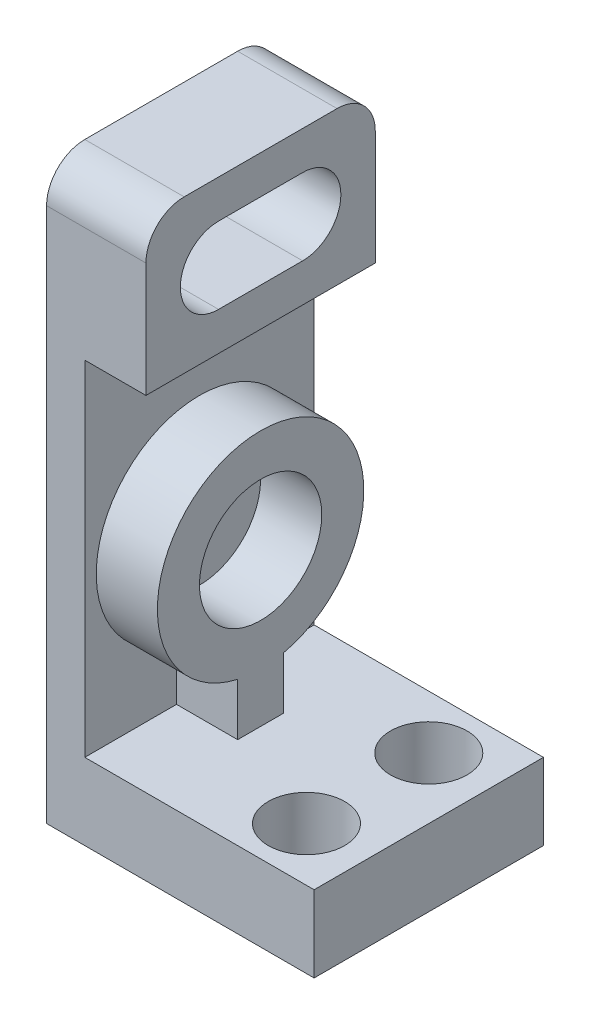
ISO-10303-21;
HEADER;
FILE_DESCRIPTION(('STEP AP214'),'2;1');
FILE_NAME('part.step','',(''),(''),'','','');
FILE_SCHEMA(('AUTOMOTIVE_DESIGN { 1 0 10303 214 1 1 1 1 }'));
ENDSEC;
DATA;
#1=APPLICATION_CONTEXT('core data for automotive mechanical design processes');
#2=APPLICATION_PROTOCOL_DEFINITION('international standard','automotive_design',2000,#1);
#3=PRODUCT_CONTEXT('',#1,'mechanical');
#4=PRODUCT('Part','Part','',(#3));
#5=PRODUCT_RELATED_PRODUCT_CATEGORY('part','',(#4));
#6=PRODUCT_DEFINITION_FORMATION('','',#4);
#7=PRODUCT_DEFINITION_CONTEXT('part definition',#1,'design');
#8=PRODUCT_DEFINITION('design','',#6,#7);
#9=PRODUCT_DEFINITION_SHAPE('','',#8);
#10=(LENGTH_UNIT() NAMED_UNIT(*) SI_UNIT(.MILLI.,.METRE.));
#11=(NAMED_UNIT(*) PLANE_ANGLE_UNIT() SI_UNIT($,.RADIAN.));
#12=(NAMED_UNIT(*) SI_UNIT($,.STERADIAN.) SOLID_ANGLE_UNIT());
#13=UNCERTAINTY_MEASURE_WITH_UNIT(LENGTH_MEASURE(1.E-05),#10,'distance_accuracy_value','');
#14=(GEOMETRIC_REPRESENTATION_CONTEXT(3) GLOBAL_UNCERTAINTY_ASSIGNED_CONTEXT((#13)) GLOBAL_UNIT_ASSIGNED_CONTEXT((#10,
#11,#12)) REPRESENTATION_CONTEXT('',''));
#15=CARTESIAN_POINT('',(0.,0.,0.));
#16=DIRECTION('',(0.,0.,1.));
#17=DIRECTION('',(1.,0.,0.));
#18=AXIS2_PLACEMENT_3D('',#15,#16,#17);
#19=CARTESIAN_POINT('',(0.,10.,-30.));
#20=DIRECTION('',(0.,1.,0.));
#21=DIRECTION('',(0.,0.,1.));
#22=AXIS2_PLACEMENT_3D('',#19,#20,#21);
#23=PLANE('',#22);
#24=CARTESIAN_POINT('',(27.,10.,-23.));
#25=DIRECTION('',(0.,1.,0.));
#26=DIRECTION('',(0.,0.,1.));
#27=AXIS2_PLACEMENT_3D('',#24,#25,#26);
#28=CIRCLE('',#27,5.);
#29=CARTESIAN_POINT('',(27.,10.,-18.));
#30=VERTEX_POINT('',#29);
#31=EDGE_CURVE('E263',#30,#30,#28,.T.);
#32=ORIENTED_EDGE('',*,*,#31,.F.);
#33=EDGE_LOOP('',(#32));
#34=FACE_BOUND('',#33,.T.);
#35=CARTESIAN_POINT('',(27.,10.,-7.));
#36=DIRECTION('',(0.,1.,0.));
#37=DIRECTION('',(0.,0.,1.));
#38=AXIS2_PLACEMENT_3D('',#35,#36,#37);
#39=CIRCLE('',#38,5.);
#40=CARTESIAN_POINT('',(27.,10.,-2.));
#41=VERTEX_POINT('',#40);
#42=EDGE_CURVE('E251',#41,#41,#39,.T.);
#43=ORIENTED_EDGE('',*,*,#42,.F.);
#44=EDGE_LOOP('',(#43));
#45=FACE_BOUND('',#44,.T.);
#46=DIRECTION('',(0.,0.,1.));
#47=VECTOR('',#46,1.);
#48=CARTESIAN_POINT('',(5.,10.,-30.));
#49=LINE('',#48,#47);
#50=CARTESIAN_POINT('',(5.,10.,-30.));
#51=VERTEX_POINT('',#50);
#52=CARTESIAN_POINT('',(5.,10.,-18.));
#53=VERTEX_POINT('',#52);
#54=EDGE_CURVE('E186',#51,#53,#49,.T.);
#55=ORIENTED_EDGE('',*,*,#54,.T.);
#56=DIRECTION('',(-1.,0.,0.));
#57=VECTOR('',#56,1.);
#58=CARTESIAN_POINT('',(13.,10.,-18.));
#59=LINE('',#58,#57);
#60=CARTESIAN_POINT('',(13.,10.,-18.));
#61=VERTEX_POINT('',#60);
#62=EDGE_CURVE('E169',#61,#53,#59,.T.);
#63=ORIENTED_EDGE('',*,*,#62,.F.);
#64=DIRECTION('',(0.,0.,-1.));
#65=VECTOR('',#64,1.);
#66=CARTESIAN_POINT('',(13.,10.,-12.));
#67=LINE('',#66,#65);
#68=CARTESIAN_POINT('',(13.,10.,-12.));
#69=VERTEX_POINT('',#68);
#70=EDGE_CURVE('E172',#69,#61,#67,.T.);
#71=ORIENTED_EDGE('',*,*,#70,.F.);
#72=DIRECTION('',(-1.,0.,0.));
#73=VECTOR('',#72,1.);
#74=CARTESIAN_POINT('',(13.,10.,-12.));
#75=LINE('',#74,#73);
#76=CARTESIAN_POINT('',(5.,10.,-12.));
#77=VERTEX_POINT('',#76);
#78=EDGE_CURVE('E371',#69,#77,#75,.T.);
#79=ORIENTED_EDGE('',*,*,#78,.T.);
#80=CARTESIAN_POINT('',(5.,10.,0.));
#81=VERTEX_POINT('',#80);
#82=EDGE_CURVE('E275',#77,#81,#49,.T.);
#83=ORIENTED_EDGE('',*,*,#82,.T.);
#84=DIRECTION('',(-1.,0.,0.));
#85=VECTOR('',#84,1.);
#86=CARTESIAN_POINT('',(0.,10.,0.));
#87=LINE('',#86,#85);
#88=CARTESIAN_POINT('',(35.,10.,0.));
#89=VERTEX_POINT('',#88);
#90=EDGE_CURVE('E288',#89,#81,#87,.T.);
#91=ORIENTED_EDGE('',*,*,#90,.F.);
#92=DIRECTION('',(0.,0.,1.));
#93=VECTOR('',#92,1.);
#94=CARTESIAN_POINT('',(35.,10.,-30.));
#95=LINE('',#94,#93);
#96=CARTESIAN_POINT('',(35.,10.,-30.));
#97=VERTEX_POINT('',#96);
#98=EDGE_CURVE('E50',#97,#89,#95,.T.);
#99=ORIENTED_EDGE('',*,*,#98,.F.);
#100=DIRECTION('',(-1.,0.,0.));
#101=VECTOR('',#100,1.);
#102=CARTESIAN_POINT('',(0.,10.,-30.));
#103=LINE('',#102,#101);
#104=EDGE_CURVE('E295',#97,#51,#103,.T.);
#105=ORIENTED_EDGE('',*,*,#104,.T.);
#106=EDGE_LOOP('',(#55,#63,#71,#79,#83,#91,#99,#105));
#107=FACE_BOUND('',#106,.T.);
#108=ADVANCED_FACE('F39',(#34,#45,#107),#23,.T.);
#109=CARTESIAN_POINT('',(0.,0.,-30.));
#110=DIRECTION('',(-1.,0.,0.));
#111=DIRECTION('',(0.,0.,1.));
#112=AXIS2_PLACEMENT_3D('',#109,#110,#111);
#113=PLANE('',#112);
#114=CARTESIAN_POINT('',(0.,65.,-9.5));
#115=DIRECTION('',(1.,0.,0.));
#116=DIRECTION('',(0.,0.,-1.));
#117=AXIS2_PLACEMENT_3D('',#114,#115,#116);
#118=CIRCLE('',#117,5.);
#119=CARTESIAN_POINT('',(0.,70.,-9.5));
#120=VERTEX_POINT('',#119);
#121=CARTESIAN_POINT('',(0.,60.,-9.5));
#122=VERTEX_POINT('',#121);
#123=EDGE_CURVE('E198',#120,#122,#118,.T.);
#124=ORIENTED_EDGE('',*,*,#123,.T.);
#125=DIRECTION('',(0.,0.,-1.));
#126=VECTOR('',#125,1.);
#127=CARTESIAN_POINT('',(0.,60.,-9.5));
#128=LINE('',#127,#126);
#129=CARTESIAN_POINT('',(0.,60.,-20.5));
#130=VERTEX_POINT('',#129);
#131=EDGE_CURVE('E200',#122,#130,#128,.T.);
#132=ORIENTED_EDGE('',*,*,#131,.T.);
#133=CARTESIAN_POINT('',(0.,65.,-20.5));
#134=DIRECTION('',(1.,0.,0.));
#135=DIRECTION('',(0.,0.,-1.));
#136=AXIS2_PLACEMENT_3D('',#133,#134,#135);
#137=CIRCLE('',#136,5.);
#138=CARTESIAN_POINT('',(0.,70.,-20.5));
#139=VERTEX_POINT('',#138);
#140=EDGE_CURVE('E65',#130,#139,#137,.T.);
#141=ORIENTED_EDGE('',*,*,#140,.T.);
#142=DIRECTION('',(0.,0.,1.));
#143=VECTOR('',#142,1.);
#144=CARTESIAN_POINT('',(0.,70.,-9.5));
#145=LINE('',#144,#143);
#146=EDGE_CURVE('E204',#139,#120,#145,.T.);
#147=ORIENTED_EDGE('',*,*,#146,.T.);
#148=EDGE_LOOP('',(#124,#132,#141,#147));
#149=FACE_BOUND('',#148,.T.);
#150=DIRECTION('',(0.,-1.,0.));
#151=VECTOR('',#150,1.);
#152=CARTESIAN_POINT('',(0.,0.,0.));
#153=LINE('',#152,#151);
#154=CARTESIAN_POINT('',(0.,70.,0.));
#155=VERTEX_POINT('',#154);
#156=CARTESIAN_POINT('',(0.,0.,0.));
#157=VERTEX_POINT('',#156);
#158=EDGE_CURVE('E278',#155,#157,#153,.T.);
#159=ORIENTED_EDGE('',*,*,#158,.F.);
#160=CARTESIAN_POINT('',(0.,70.,-5.));
#161=DIRECTION('',(1.,0.,0.));
#162=DIRECTION('',(0.,0.,1.));
#163=AXIS2_PLACEMENT_3D('',#160,#161,#162);
#164=CIRCLE('',#163,5.);
#165=CARTESIAN_POINT('',(0.,75.,-5.00000000000004));
#166=VERTEX_POINT('',#165);
#167=EDGE_CURVE('E249',#166,#155,#164,.T.);
#168=ORIENTED_EDGE('',*,*,#167,.F.);
#169=DIRECTION('',(0.,0.,1.));
#170=VECTOR('',#169,1.);
#171=CARTESIAN_POINT('',(0.,75.,-5.00000000000004));
#172=LINE('',#171,#170);
#173=CARTESIAN_POINT('',(0.,75.,-25.));
#174=VERTEX_POINT('',#173);
#175=EDGE_CURVE('E244',#174,#166,#172,.T.);
#176=ORIENTED_EDGE('',*,*,#175,.F.);
#177=CARTESIAN_POINT('',(0.,70.,-25.));
#178=DIRECTION('',(1.,0.,0.));
#179=DIRECTION('',(0.,0.,1.));
#180=AXIS2_PLACEMENT_3D('',#177,#178,#179);
#181=CIRCLE('',#180,5.);
#182=CARTESIAN_POINT('',(0.,70.,-30.));
#183=VERTEX_POINT('',#182);
#184=EDGE_CURVE('E243',#183,#174,#181,.T.);
#185=ORIENTED_EDGE('',*,*,#184,.F.);
#186=DIRECTION('',(0.,-1.,0.));
#187=VECTOR('',#186,1.);
#188=CARTESIAN_POINT('',(0.,0.,-30.));
#189=LINE('',#188,#187);
#190=CARTESIAN_POINT('',(0.,0.,-30.));
#191=VERTEX_POINT('',#190);
#192=EDGE_CURVE('E285',#183,#191,#189,.T.);
#193=ORIENTED_EDGE('',*,*,#192,.T.);
#194=DIRECTION('',(0.,0.,1.));
#195=VECTOR('',#194,1.);
#196=CARTESIAN_POINT('',(0.,0.,-30.));
#197=LINE('',#196,#195);
#198=EDGE_CURVE('E294',#191,#157,#197,.T.);
#199=ORIENTED_EDGE('',*,*,#198,.T.);
#200=EDGE_LOOP('',(#159,#168,#176,#185,#193,#199));
#201=FACE_BOUND('',#200,.T.);
#202=ADVANCED_FACE('F41',(#149,#201),#113,.T.);
#203=CARTESIAN_POINT('',(35.,0.,-30.));
#204=DIRECTION('',(1.,0.,0.));
#205=DIRECTION('',(0.,0.,-1.));
#206=AXIS2_PLACEMENT_3D('',#203,#204,#205);
#207=PLANE('',#206);
#208=DIRECTION('',(0.,1.,0.));
#209=VECTOR('',#208,1.);
#210=CARTESIAN_POINT('',(35.,0.,0.));
#211=LINE('',#210,#209);
#212=CARTESIAN_POINT('',(35.,0.,0.));
#213=VERTEX_POINT('',#212);
#214=EDGE_CURVE('E297',#213,#89,#211,.T.);
#215=ORIENTED_EDGE('',*,*,#214,.F.);
#216=DIRECTION('',(0.,0.,1.));
#217=VECTOR('',#216,1.);
#218=CARTESIAN_POINT('',(35.,0.,-30.));
#219=LINE('',#218,#217);
#220=CARTESIAN_POINT('',(35.,0.,-30.));
#221=VERTEX_POINT('',#220);
#222=EDGE_CURVE('E308',#221,#213,#219,.T.);
#223=ORIENTED_EDGE('',*,*,#222,.F.);
#224=DIRECTION('',(0.,1.,0.));
#225=VECTOR('',#224,1.);
#226=CARTESIAN_POINT('',(35.,0.,-30.));
#227=LINE('',#226,#225);
#228=EDGE_CURVE('E290',#221,#97,#227,.T.);
#229=ORIENTED_EDGE('',*,*,#228,.T.);
#230=ORIENTED_EDGE('',*,*,#98,.T.);
#231=EDGE_LOOP('',(#215,#223,#229,#230));
#232=FACE_BOUND('',#231,.T.);
#233=ADVANCED_FACE('F319',(#232),#207,.T.);
#234=CARTESIAN_POINT('',(0.,0.,-30.));
#235=DIRECTION('',(0.,-1.,0.));
#236=DIRECTION('',(0.,0.,-1.));
#237=AXIS2_PLACEMENT_3D('',#234,#235,#236);
#238=PLANE('',#237);
#239=CARTESIAN_POINT('',(27.,0.,-23.));
#240=DIRECTION('',(0.,-1.,0.));
#241=DIRECTION('',(0.,0.,-1.));
#242=AXIS2_PLACEMENT_3D('',#239,#240,#241);
#243=CIRCLE('',#242,5.);
#244=CARTESIAN_POINT('',(27.,0.,-28.));
#245=VERTEX_POINT('',#244);
#246=EDGE_CURVE('E277',#245,#245,#243,.T.);
#247=ORIENTED_EDGE('',*,*,#246,.F.);
#248=EDGE_LOOP('',(#247));
#249=FACE_BOUND('',#248,.T.);
#250=CARTESIAN_POINT('',(27.,0.,-7.));
#251=DIRECTION('',(0.,-1.,0.));
#252=DIRECTION('',(0.,0.,-1.));
#253=AXIS2_PLACEMENT_3D('',#250,#251,#252);
#254=CIRCLE('',#253,5.);
#255=CARTESIAN_POINT('',(27.,0.,-12.));
#256=VERTEX_POINT('',#255);
#257=EDGE_CURVE('E266',#256,#256,#254,.T.);
#258=ORIENTED_EDGE('',*,*,#257,.F.);
#259=EDGE_LOOP('',(#258));
#260=FACE_BOUND('',#259,.T.);
#261=DIRECTION('',(1.,0.,0.));
#262=VECTOR('',#261,1.);
#263=CARTESIAN_POINT('',(0.,0.,0.));
#264=LINE('',#263,#262);
#265=EDGE_CURVE('E300',#157,#213,#264,.T.);
#266=ORIENTED_EDGE('',*,*,#265,.F.);
#267=ORIENTED_EDGE('',*,*,#198,.F.);
#268=DIRECTION('',(1.,0.,0.));
#269=VECTOR('',#268,1.);
#270=CARTESIAN_POINT('',(0.,0.,-30.));
#271=LINE('',#270,#269);
#272=EDGE_CURVE('E282',#191,#221,#271,.T.);
#273=ORIENTED_EDGE('',*,*,#272,.T.);
#274=ORIENTED_EDGE('',*,*,#222,.T.);
#275=EDGE_LOOP('',(#266,#267,#273,#274));
#276=FACE_BOUND('',#275,.T.);
#277=ADVANCED_FACE('F316',(#249,#260,#276),#238,.T.);
#278=CARTESIAN_POINT('',(0.,0.,-30.));
#279=DIRECTION('',(0.,0.,-1.));
#280=DIRECTION('',(-1.,0.,0.));
#281=AXIS2_PLACEMENT_3D('',#278,#279,#280);
#282=PLANE('',#281);
#283=ORIENTED_EDGE('',*,*,#192,.F.);
#284=DIRECTION('',(1.,0.,0.));
#285=VECTOR('',#284,1.);
#286=CARTESIAN_POINT('',(0.,70.,-30.));
#287=LINE('',#286,#285);
#288=CARTESIAN_POINT('',(13.,70.,-30.));
#289=VERTEX_POINT('',#288);
#290=EDGE_CURVE('E256',#183,#289,#287,.T.);
#291=ORIENTED_EDGE('',*,*,#290,.T.);
#292=DIRECTION('',(0.,1.,0.));
#293=VECTOR('',#292,1.);
#294=CARTESIAN_POINT('',(13.,55.,-30.));
#295=LINE('',#294,#293);
#296=CARTESIAN_POINT('',(13.,55.,-30.));
#297=VERTEX_POINT('',#296);
#298=EDGE_CURVE('E229',#297,#289,#295,.T.);
#299=ORIENTED_EDGE('',*,*,#298,.F.);
#300=DIRECTION('',(1.,0.,0.));
#301=VECTOR('',#300,1.);
#302=CARTESIAN_POINT('',(0.,55.,-30.));
#303=LINE('',#302,#301);
#304=CARTESIAN_POINT('',(5.,55.,-30.));
#305=VERTEX_POINT('',#304);
#306=EDGE_CURVE('E257',#305,#297,#303,.T.);
#307=ORIENTED_EDGE('',*,*,#306,.F.);
#308=DIRECTION('',(0.,1.,0.));
#309=VECTOR('',#308,1.);
#310=CARTESIAN_POINT('',(5.,10.,-30.));
#311=LINE('',#310,#309);
#312=EDGE_CURVE('E267',#51,#305,#311,.T.);
#313=ORIENTED_EDGE('',*,*,#312,.F.);
#314=ORIENTED_EDGE('',*,*,#104,.F.);
#315=ORIENTED_EDGE('',*,*,#228,.F.);
#316=ORIENTED_EDGE('',*,*,#272,.F.);
#317=EDGE_LOOP('',(#283,#291,#299,#307,#313,#314,#315,#316));
#318=FACE_BOUND('',#317,.T.);
#319=ADVANCED_FACE('F317',(#318),#282,.T.);
#320=CARTESIAN_POINT('',(0.,0.,0.));
#321=DIRECTION('',(0.,0.,-1.));
#322=DIRECTION('',(-1.,0.,0.));
#323=AXIS2_PLACEMENT_3D('',#320,#321,#322);
#324=PLANE('',#323);
#325=ORIENTED_EDGE('',*,*,#158,.T.);
#326=ORIENTED_EDGE('',*,*,#265,.T.);
#327=ORIENTED_EDGE('',*,*,#214,.T.);
#328=ORIENTED_EDGE('',*,*,#90,.T.);
#329=DIRECTION('',(0.,1.,0.));
#330=VECTOR('',#329,1.);
#331=CARTESIAN_POINT('',(5.,10.,0.));
#332=LINE('',#331,#330);
#333=CARTESIAN_POINT('',(5.,55.,0.));
#334=VERTEX_POINT('',#333);
#335=EDGE_CURVE('E272',#81,#334,#332,.T.);
#336=ORIENTED_EDGE('',*,*,#335,.T.);
#337=DIRECTION('',(1.,0.,0.));
#338=VECTOR('',#337,1.);
#339=CARTESIAN_POINT('',(0.,55.,0.));
#340=LINE('',#339,#338);
#341=CARTESIAN_POINT('',(13.,55.,0.));
#342=VERTEX_POINT('',#341);
#343=EDGE_CURVE('E246',#334,#342,#340,.T.);
#344=ORIENTED_EDGE('',*,*,#343,.T.);
#345=DIRECTION('',(0.,-1.,0.));
#346=VECTOR('',#345,1.);
#347=CARTESIAN_POINT('',(13.,55.,0.));
#348=LINE('',#347,#346);
#349=CARTESIAN_POINT('',(13.,70.,0.));
#350=VERTEX_POINT('',#349);
#351=EDGE_CURVE('E220',#350,#342,#348,.T.);
#352=ORIENTED_EDGE('',*,*,#351,.F.);
#353=DIRECTION('',(1.,0.,0.));
#354=VECTOR('',#353,1.);
#355=CARTESIAN_POINT('',(0.,70.,0.));
#356=LINE('',#355,#354);
#357=EDGE_CURVE('E253',#155,#350,#356,.T.);
#358=ORIENTED_EDGE('',*,*,#357,.F.);
#359=EDGE_LOOP('',(#325,#326,#327,#328,#336,#344,#352,#358));
#360=FACE_BOUND('',#359,.T.);
#361=ADVANCED_FACE('F327',(#360),#324,.F.);
#362=CARTESIAN_POINT('',(5.,10.,-30.));
#363=DIRECTION('',(1.,0.,0.));
#364=DIRECTION('',(0.,0.,-1.));
#365=AXIS2_PLACEMENT_3D('',#362,#363,#364);
#366=PLANE('',#365);
#367=CARTESIAN_POINT('',(5.,30.,-15.));
#368=DIRECTION('',(1.,0.,0.));
#369=DIRECTION('',(0.,0.,-1.));
#370=AXIS2_PLACEMENT_3D('',#367,#368,#369);
#371=CIRCLE('',#370,13.5);
#372=CARTESIAN_POINT('',(5.,16.8375534189118,-18.));
#373=VERTEX_POINT('',#372);
#374=CARTESIAN_POINT('',(5.,16.8375534189118,-12.));
#375=VERTEX_POINT('',#374);
#376=EDGE_CURVE('E363',#373,#375,#371,.T.);
#377=ORIENTED_EDGE('',*,*,#376,.F.);
#378=DIRECTION('',(0.,1.,0.));
#379=VECTOR('',#378,1.);
#380=CARTESIAN_POINT('',(5.,16.8375534189118,-18.));
#381=LINE('',#380,#379);
#382=EDGE_CURVE('E360',#53,#373,#381,.T.);
#383=ORIENTED_EDGE('',*,*,#382,.F.);
#384=ORIENTED_EDGE('',*,*,#54,.F.);
#385=ORIENTED_EDGE('',*,*,#312,.T.);
#386=DIRECTION('',(0.,0.,1.));
#387=VECTOR('',#386,1.);
#388=CARTESIAN_POINT('',(5.,55.,-30.));
#389=LINE('',#388,#387);
#390=EDGE_CURVE('E280',#305,#334,#389,.T.);
#391=ORIENTED_EDGE('',*,*,#390,.T.);
#392=ORIENTED_EDGE('',*,*,#335,.F.);
#393=ORIENTED_EDGE('',*,*,#82,.F.);
#394=DIRECTION('',(0.,-1.,0.));
#395=VECTOR('',#394,1.);
#396=CARTESIAN_POINT('',(5.,16.8375534189118,-12.));
#397=LINE('',#396,#395);
#398=EDGE_CURVE('E184',#375,#77,#397,.T.);
#399=ORIENTED_EDGE('',*,*,#398,.F.);
#400=EDGE_LOOP('',(#377,#383,#384,#385,#391,#392,#393,#399));
#401=FACE_BOUND('',#400,.T.);
#402=ADVANCED_FACE('F357',(#401),#366,.T.);
#403=CARTESIAN_POINT('',(27.,-20.,-7.));
#404=DIRECTION('',(0.,1.,0.));
#405=DIRECTION('',(0.,0.,1.));
#406=AXIS2_PLACEMENT_3D('',#403,#404,#405);
#407=CYLINDRICAL_SURFACE('',#406,5.);
#408=ORIENTED_EDGE('',*,*,#257,.T.);
#409=EDGE_LOOP('',(#408));
#410=FACE_BOUND('',#409,.T.);
#411=ORIENTED_EDGE('',*,*,#42,.T.);
#412=EDGE_LOOP('',(#411));
#413=FACE_BOUND('',#412,.T.);
#414=ADVANCED_FACE('F400',(#410,#413),#407,.F.);
#415=CARTESIAN_POINT('',(27.,-20.,-23.));
#416=DIRECTION('',(0.,1.,0.));
#417=DIRECTION('',(0.,0.,1.));
#418=AXIS2_PLACEMENT_3D('',#415,#416,#417);
#419=CYLINDRICAL_SURFACE('',#418,5.);
#420=ORIENTED_EDGE('',*,*,#246,.T.);
#421=EDGE_LOOP('',(#420));
#422=FACE_BOUND('',#421,.T.);
#423=ORIENTED_EDGE('',*,*,#31,.T.);
#424=EDGE_LOOP('',(#423));
#425=FACE_BOUND('',#424,.T.);
#426=ADVANCED_FACE('F311',(#422,#425),#419,.F.);
#427=CARTESIAN_POINT('',(0.,55.,0.));
#428=DIRECTION('',(0.,-1.,0.));
#429=DIRECTION('',(0.,0.,-1.));
#430=AXIS2_PLACEMENT_3D('',#427,#428,#429);
#431=PLANE('',#430);
#432=ORIENTED_EDGE('',*,*,#390,.F.);
#433=ORIENTED_EDGE('',*,*,#306,.T.);
#434=DIRECTION('',(0.,0.,-1.));
#435=VECTOR('',#434,1.);
#436=CARTESIAN_POINT('',(13.,55.,0.));
#437=LINE('',#436,#435);
#438=EDGE_CURVE('E228',#342,#297,#437,.T.);
#439=ORIENTED_EDGE('',*,*,#438,.F.);
#440=ORIENTED_EDGE('',*,*,#343,.F.);
#441=EDGE_LOOP('',(#432,#433,#439,#440));
#442=FACE_BOUND('',#441,.T.);
#443=ADVANCED_FACE('F355',(#442),#431,.T.);
#444=CARTESIAN_POINT('',(0.,70.,-5.));
#445=DIRECTION('',(1.,0.,0.));
#446=DIRECTION('',(0.,0.,-1.));
#447=AXIS2_PLACEMENT_3D('',#444,#445,#446);
#448=CYLINDRICAL_SURFACE('',#447,5.);
#449=ORIENTED_EDGE('',*,*,#357,.T.);
#450=CARTESIAN_POINT('',(13.,70.,-5.));
#451=DIRECTION('',(1.,0.,0.));
#452=DIRECTION('',(0.,0.,1.));
#453=AXIS2_PLACEMENT_3D('',#450,#451,#452);
#454=CIRCLE('',#453,5.);
#455=CARTESIAN_POINT('',(13.,75.,-5.00000000000004));
#456=VERTEX_POINT('',#455);
#457=EDGE_CURVE('E236',#456,#350,#454,.T.);
#458=ORIENTED_EDGE('',*,*,#457,.F.);
#459=DIRECTION('',(1.,0.,0.));
#460=VECTOR('',#459,1.);
#461=CARTESIAN_POINT('',(0.,75.,-5.00000000000004));
#462=LINE('',#461,#460);
#463=EDGE_CURVE('E255',#166,#456,#462,.T.);
#464=ORIENTED_EDGE('',*,*,#463,.F.);
#465=ORIENTED_EDGE('',*,*,#167,.T.);
#466=EDGE_LOOP('',(#449,#458,#464,#465));
#467=FACE_BOUND('',#466,.T.);
#468=ADVANCED_FACE('F346',(#467),#448,.T.);
#469=CARTESIAN_POINT('',(0.,75.,-5.00000000000004));
#470=DIRECTION('',(0.,1.,0.));
#471=DIRECTION('',(0.,0.,1.));
#472=AXIS2_PLACEMENT_3D('',#469,#470,#471);
#473=PLANE('',#472);
#474=ORIENTED_EDGE('',*,*,#463,.T.);
#475=DIRECTION('',(0.,0.,1.));
#476=VECTOR('',#475,1.);
#477=CARTESIAN_POINT('',(13.,75.,-5.00000000000004));
#478=LINE('',#477,#476);
#479=CARTESIAN_POINT('',(13.,75.,-25.));
#480=VERTEX_POINT('',#479);
#481=EDGE_CURVE('E231',#480,#456,#478,.T.);
#482=ORIENTED_EDGE('',*,*,#481,.F.);
#483=DIRECTION('',(1.,0.,0.));
#484=VECTOR('',#483,1.);
#485=CARTESIAN_POINT('',(0.,75.,-25.));
#486=LINE('',#485,#484);
#487=EDGE_CURVE('E258',#174,#480,#486,.T.);
#488=ORIENTED_EDGE('',*,*,#487,.F.);
#489=ORIENTED_EDGE('',*,*,#175,.T.);
#490=EDGE_LOOP('',(#474,#482,#488,#489));
#491=FACE_BOUND('',#490,.T.);
#492=ADVANCED_FACE('F347',(#491),#473,.T.);
#493=CARTESIAN_POINT('',(0.,70.,-25.));
#494=DIRECTION('',(1.,0.,0.));
#495=DIRECTION('',(0.,0.,-1.));
#496=AXIS2_PLACEMENT_3D('',#493,#494,#495);
#497=CYLINDRICAL_SURFACE('',#496,5.);
#498=ORIENTED_EDGE('',*,*,#487,.T.);
#499=CARTESIAN_POINT('',(13.,70.,-25.));
#500=DIRECTION('',(1.,0.,0.));
#501=DIRECTION('',(0.,0.,1.));
#502=AXIS2_PLACEMENT_3D('',#499,#500,#501);
#503=CIRCLE('',#502,5.);
#504=EDGE_CURVE('E234',#289,#480,#503,.T.);
#505=ORIENTED_EDGE('',*,*,#504,.F.);
#506=ORIENTED_EDGE('',*,*,#290,.F.);
#507=ORIENTED_EDGE('',*,*,#184,.T.);
#508=EDGE_LOOP('',(#498,#505,#506,#507));
#509=FACE_BOUND('',#508,.T.);
#510=ADVANCED_FACE('F337',(#509),#497,.T.);
#511=CARTESIAN_POINT('',(13.,70.,-5.));
#512=DIRECTION('',(-1.,0.,0.));
#513=DIRECTION('',(0.,0.,1.));
#514=AXIS2_PLACEMENT_3D('',#511,#512,#513);
#515=PLANE('',#514);
#516=DIRECTION('',(0.,0.,-1.));
#517=VECTOR('',#516,1.);
#518=CARTESIAN_POINT('',(13.,60.,-9.5));
#519=LINE('',#518,#517);
#520=CARTESIAN_POINT('',(13.,60.,-9.5));
#521=VERTEX_POINT('',#520);
#522=CARTESIAN_POINT('',(13.,60.,-20.5));
#523=VERTEX_POINT('',#522);
#524=EDGE_CURVE('E193',#521,#523,#519,.T.);
#525=ORIENTED_EDGE('',*,*,#524,.F.);
#526=CARTESIAN_POINT('',(13.,65.,-9.5));
#527=DIRECTION('',(1.,0.,0.));
#528=DIRECTION('',(0.,0.,-1.));
#529=AXIS2_PLACEMENT_3D('',#526,#527,#528);
#530=CIRCLE('',#529,5.);
#531=CARTESIAN_POINT('',(13.,70.,-9.5));
#532=VERTEX_POINT('',#531);
#533=EDGE_CURVE('E189',#532,#521,#530,.T.);
#534=ORIENTED_EDGE('',*,*,#533,.F.);
#535=DIRECTION('',(0.,0.,1.));
#536=VECTOR('',#535,1.);
#537=CARTESIAN_POINT('',(13.,70.,-9.5));
#538=LINE('',#537,#536);
#539=CARTESIAN_POINT('',(13.,70.,-20.5));
#540=VERTEX_POINT('',#539);
#541=EDGE_CURVE('E199',#540,#532,#538,.T.);
#542=ORIENTED_EDGE('',*,*,#541,.F.);
#543=CARTESIAN_POINT('',(13.,65.,-20.5));
#544=DIRECTION('',(1.,0.,0.));
#545=DIRECTION('',(0.,0.,-1.));
#546=AXIS2_PLACEMENT_3D('',#543,#544,#545);
#547=CIRCLE('',#546,5.);
#548=EDGE_CURVE('E209',#523,#540,#547,.T.);
#549=ORIENTED_EDGE('',*,*,#548,.F.);
#550=EDGE_LOOP('',(#525,#534,#542,#549));
#551=FACE_BOUND('',#550,.T.);
#552=ORIENTED_EDGE('',*,*,#351,.T.);
#553=ORIENTED_EDGE('',*,*,#438,.T.);
#554=ORIENTED_EDGE('',*,*,#298,.T.);
#555=ORIENTED_EDGE('',*,*,#504,.T.);
#556=ORIENTED_EDGE('',*,*,#481,.T.);
#557=ORIENTED_EDGE('',*,*,#457,.T.);
#558=EDGE_LOOP('',(#552,#553,#554,#555,#556,#557));
#559=FACE_BOUND('',#558,.T.);
#560=ADVANCED_FACE('F342',(#551,#559),#515,.F.);
#561=CARTESIAN_POINT('',(0.,65.,-9.5));
#562=DIRECTION('',(1.,0.,0.));
#563=DIRECTION('',(0.,0.,-1.));
#564=AXIS2_PLACEMENT_3D('',#561,#562,#563);
#565=CYLINDRICAL_SURFACE('',#564,5.);
#566=ORIENTED_EDGE('',*,*,#533,.T.);
#567=DIRECTION('',(1.,0.,0.));
#568=VECTOR('',#567,1.);
#569=CARTESIAN_POINT('',(0.,60.,-9.5));
#570=LINE('',#569,#568);
#571=EDGE_CURVE('E206',#122,#521,#570,.T.);
#572=ORIENTED_EDGE('',*,*,#571,.F.);
#573=ORIENTED_EDGE('',*,*,#123,.F.);
#574=DIRECTION('',(1.,0.,0.));
#575=VECTOR('',#574,1.);
#576=CARTESIAN_POINT('',(0.,70.,-9.5));
#577=LINE('',#576,#575);
#578=EDGE_CURVE('E214',#120,#532,#577,.T.);
#579=ORIENTED_EDGE('',*,*,#578,.T.);
#580=EDGE_LOOP('',(#566,#572,#573,#579));
#581=FACE_BOUND('',#580,.T.);
#582=ADVANCED_FACE('F418',(#581),#565,.F.);
#583=CARTESIAN_POINT('',(0.,70.,-9.5));
#584=DIRECTION('',(0.,1.,0.));
#585=DIRECTION('',(0.,0.,1.));
#586=AXIS2_PLACEMENT_3D('',#583,#584,#585);
#587=PLANE('',#586);
#588=ORIENTED_EDGE('',*,*,#541,.T.);
#589=ORIENTED_EDGE('',*,*,#578,.F.);
#590=ORIENTED_EDGE('',*,*,#146,.F.);
#591=DIRECTION('',(1.,0.,0.));
#592=VECTOR('',#591,1.);
#593=CARTESIAN_POINT('',(0.,70.,-20.5));
#594=LINE('',#593,#592);
#595=EDGE_CURVE('E217',#139,#540,#594,.T.);
#596=ORIENTED_EDGE('',*,*,#595,.T.);
#597=EDGE_LOOP('',(#588,#589,#590,#596));
#598=FACE_BOUND('',#597,.T.);
#599=ADVANCED_FACE('F419',(#598),#587,.F.);
#600=CARTESIAN_POINT('',(0.,65.,-20.5));
#601=DIRECTION('',(1.,0.,0.));
#602=DIRECTION('',(0.,0.,-1.));
#603=AXIS2_PLACEMENT_3D('',#600,#601,#602);
#604=CYLINDRICAL_SURFACE('',#603,5.);
#605=ORIENTED_EDGE('',*,*,#548,.T.);
#606=ORIENTED_EDGE('',*,*,#595,.F.);
#607=ORIENTED_EDGE('',*,*,#140,.F.);
#608=DIRECTION('',(1.,0.,0.));
#609=VECTOR('',#608,1.);
#610=CARTESIAN_POINT('',(0.,60.,-20.5));
#611=LINE('',#610,#609);
#612=EDGE_CURVE('E219',#130,#523,#611,.T.);
#613=ORIENTED_EDGE('',*,*,#612,.T.);
#614=EDGE_LOOP('',(#605,#606,#607,#613));
#615=FACE_BOUND('',#614,.T.);
#616=ADVANCED_FACE('F424',(#615),#604,.F.);
#617=CARTESIAN_POINT('',(0.,60.,-9.5));
#618=DIRECTION('',(0.,-1.,0.));
#619=DIRECTION('',(0.,0.,-1.));
#620=AXIS2_PLACEMENT_3D('',#617,#618,#619);
#621=PLANE('',#620);
#622=ORIENTED_EDGE('',*,*,#524,.T.);
#623=ORIENTED_EDGE('',*,*,#612,.F.);
#624=ORIENTED_EDGE('',*,*,#131,.F.);
#625=ORIENTED_EDGE('',*,*,#571,.T.);
#626=EDGE_LOOP('',(#622,#623,#624,#625));
#627=FACE_BOUND('',#626,.T.);
#628=ADVANCED_FACE('F425',(#627),#621,.F.);
#629=CARTESIAN_POINT('',(13.,30.,-15.));
#630=DIRECTION('',(1.,0.,0.));
#631=DIRECTION('',(0.,0.,-1.));
#632=AXIS2_PLACEMENT_3D('',#629,#630,#631);
#633=PLANE('',#632);
#634=ORIENTED_EDGE('',*,*,#70,.T.);
#635=DIRECTION('',(0.,1.,0.));
#636=VECTOR('',#635,1.);
#637=CARTESIAN_POINT('',(13.,16.8375534189118,-18.));
#638=LINE('',#637,#636);
#639=CARTESIAN_POINT('',(13.,16.8375534189118,-18.));
#640=VERTEX_POINT('',#639);
#641=EDGE_CURVE('E163',#61,#640,#638,.T.);
#642=ORIENTED_EDGE('',*,*,#641,.T.);
#643=CARTESIAN_POINT('',(13.,30.,-15.));
#644=DIRECTION('',(1.,0.,0.));
#645=DIRECTION('',(0.,0.,-1.));
#646=AXIS2_PLACEMENT_3D('',#643,#644,#645);
#647=CIRCLE('',#646,13.5);
#648=CARTESIAN_POINT('',(13.,16.8375534189118,-12.));
#649=VERTEX_POINT('',#648);
#650=EDGE_CURVE('E174',#640,#649,#647,.T.);
#651=ORIENTED_EDGE('',*,*,#650,.T.);
#652=DIRECTION('',(0.,-1.,0.));
#653=VECTOR('',#652,1.);
#654=CARTESIAN_POINT('',(13.,16.8375534189118,-12.));
#655=LINE('',#654,#653);
#656=EDGE_CURVE('E176',#649,#69,#655,.T.);
#657=ORIENTED_EDGE('',*,*,#656,.T.);
#658=EDGE_LOOP('',(#634,#642,#651,#657));
#659=FACE_BOUND('',#658,.T.);
#660=CARTESIAN_POINT('',(13.,30.,-15.));
#661=DIRECTION('',(1.,0.,0.));
#662=DIRECTION('',(0.,0.,-1.));
#663=AXIS2_PLACEMENT_3D('',#660,#661,#662);
#664=CIRCLE('',#663,8.);
#665=CARTESIAN_POINT('',(13.,30.,-23.));
#666=VERTEX_POINT('',#665);
#667=EDGE_CURVE('E362',#666,#666,#664,.T.);
#668=ORIENTED_EDGE('',*,*,#667,.F.);
#669=EDGE_LOOP('',(#668));
#670=FACE_BOUND('',#669,.T.);
#671=ADVANCED_FACE('F177',(#659,#670),#633,.T.);
#672=CARTESIAN_POINT('',(13.,16.8375534189118,-18.));
#673=DIRECTION('',(0.,0.,1.));
#674=DIRECTION('',(1.,0.,0.));
#675=AXIS2_PLACEMENT_3D('',#672,#673,#674);
#676=PLANE('',#675);
#677=ORIENTED_EDGE('',*,*,#382,.T.);
#678=DIRECTION('',(-1.,0.,0.));
#679=VECTOR('',#678,1.);
#680=CARTESIAN_POINT('',(13.,16.8375534189118,-18.));
#681=LINE('',#680,#679);
#682=EDGE_CURVE('E173',#640,#373,#681,.T.);
#683=ORIENTED_EDGE('',*,*,#682,.F.);
#684=ORIENTED_EDGE('',*,*,#641,.F.);
#685=ORIENTED_EDGE('',*,*,#62,.T.);
#686=EDGE_LOOP('',(#677,#683,#684,#685));
#687=FACE_BOUND('',#686,.T.);
#688=ADVANCED_FACE('F167',(#687),#676,.F.);
#689=CARTESIAN_POINT('',(13.,30.,-15.));
#690=DIRECTION('',(-1.,0.,0.));
#691=DIRECTION('',(0.,0.,1.));
#692=AXIS2_PLACEMENT_3D('',#689,#690,#691);
#693=CYLINDRICAL_SURFACE('',#692,13.5);
#694=ORIENTED_EDGE('',*,*,#376,.T.);
#695=DIRECTION('',(-1.,0.,0.));
#696=VECTOR('',#695,1.);
#697=CARTESIAN_POINT('',(13.,16.8375534189118,-12.));
#698=LINE('',#697,#696);
#699=EDGE_CURVE('E53',#649,#375,#698,.T.);
#700=ORIENTED_EDGE('',*,*,#699,.F.);
#701=ORIENTED_EDGE('',*,*,#650,.F.);
#702=ORIENTED_EDGE('',*,*,#682,.T.);
#703=EDGE_LOOP('',(#694,#700,#701,#702));
#704=FACE_BOUND('',#703,.T.);
#705=ADVANCED_FACE('F372',(#704),#693,.T.);
#706=CARTESIAN_POINT('',(13.,16.8375534189118,-12.));
#707=DIRECTION('',(0.,0.,-1.));
#708=DIRECTION('',(-1.,0.,0.));
#709=AXIS2_PLACEMENT_3D('',#706,#707,#708);
#710=PLANE('',#709);
#711=ORIENTED_EDGE('',*,*,#398,.T.);
#712=ORIENTED_EDGE('',*,*,#78,.F.);
#713=ORIENTED_EDGE('',*,*,#656,.F.);
#714=ORIENTED_EDGE('',*,*,#699,.T.);
#715=EDGE_LOOP('',(#711,#712,#713,#714));
#716=FACE_BOUND('',#715,.T.);
#717=ADVANCED_FACE('F374',(#716),#710,.F.);
#718=CARTESIAN_POINT('',(13.,30.,-15.));
#719=DIRECTION('',(-1.,0.,0.));
#720=DIRECTION('',(0.,0.,1.));
#721=AXIS2_PLACEMENT_3D('',#718,#719,#720);
#722=CYLINDRICAL_SURFACE('',#721,8.);
#723=ORIENTED_EDGE('',*,*,#667,.T.);
#724=EDGE_LOOP('',(#723));
#725=FACE_BOUND('',#724,.T.);
#726=CARTESIAN_POINT('',(5.,30.,-15.));
#727=DIRECTION('',(1.,0.,0.));
#728=DIRECTION('',(0.,0.,-1.));
#729=AXIS2_PLACEMENT_3D('',#726,#727,#728);
#730=CIRCLE('',#729,8.);
#731=CARTESIAN_POINT('',(5.,30.,-23.));
#732=VERTEX_POINT('',#731);
#733=EDGE_CURVE('E11',#732,#732,#730,.F.);
#734=ORIENTED_EDGE('',*,*,#733,.T.);
#735=EDGE_LOOP('',(#734));
#736=FACE_BOUND('',#735,.T.);
#737=ADVANCED_FACE('F440',(#725,#736),#722,.F.);
#738=ORIENTED_EDGE('',*,*,#733,.F.);
#739=EDGE_LOOP('',(#738));
#740=FACE_BOUND('',#739,.T.);
#741=ADVANCED_FACE('F396',(#740),#366,.T.);
#742=CLOSED_SHELL('',(#108,#202,#233,#277,#319,#361,#402,#414,#426,#443,#468,#492,#510,#560,
#582,#599,#616,#628,#671,#688,#705,#717,#737,#741));
#743=MANIFOLD_SOLID_BREP('B2',#742);
#744=ADVANCED_BREP_SHAPE_REPRESENTATION('',(#18,#743),#14);
#745=SHAPE_DEFINITION_REPRESENTATION(#9,#744);
ENDSEC;
END-ISO-10303-21;
